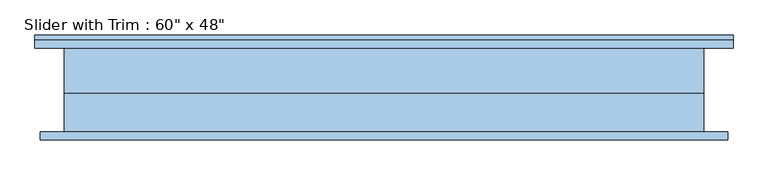
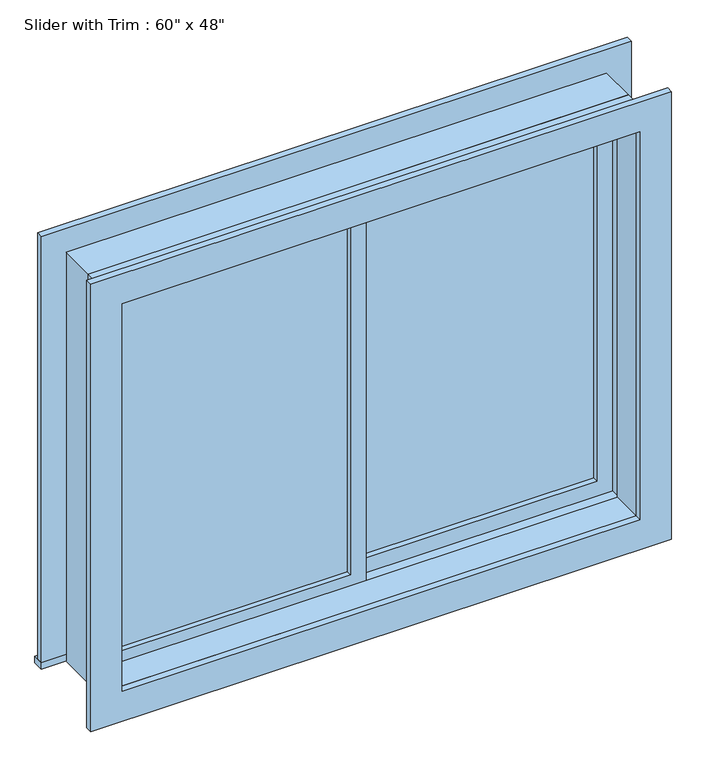
"""IFC4 building model written with IfcOpenShell, lengths in millimetres: window geometry."""

from ifc_helpers import new_model, si_unit, frame, origin, place, context, project, spatial, polyline, outline, extrude, source, transform, mapped, element, save


def window_c4d7a2b1(model_context):
    return source(origin(), model_context, "Body", "SweptSolid", [
        extrude(outline(polyline([(-698.5, 20.625), (-22.225, 20.625), (-22.225, 7.925), (-698.5, 7.925), (-698.5, 20.625)])), frame((0.0, 0.0, 977.9), z_axis=(0.0, 0.0, 1.0), x_axis=(1.0, 0.0, 0.0)), (0.0, 0.0, 1.0), 1092.2),
        extrude(outline(polyline([(2114.55, -742.95), (933.45, -742.95), (933.45, 22.225), (2114.55, 22.225), (2114.55, -742.95)]), holes=[polyline([(2070.1, -698.5), (2070.1, -22.225), (977.9, -22.225), (977.9, -698.5), (2070.1, -698.5)])]), frame((0.0, -7.95, 0.0), z_axis=(0.0, 1.0, 0.0), x_axis=(0.0, 0.0, 1.0)), (0.0, 0.0, 1.0), 44.45),
        extrude(outline(polyline([(-831.85, 131.75), (831.85, 131.75), (831.85, 100.0), (-831.85, 100.0), (-831.85, 131.75)])), frame((0.0, 0.0, 914.4), z_axis=(0.0, 0.0, 1.0), x_axis=(1.0, 0.0, 0.0)), (0.0, 0.0, 1.0), 19.05),
        extrude(outline(polyline([(2114.55, -742.95), (2114.55, 742.95), (933.45, 742.95), (933.45, 831.85), (2203.45, 831.85), (2203.45, -831.85), (933.45, -831.85), (933.45, -742.95), (2114.55, -742.95)])), frame((0.0, 100.0, 0.0), z_axis=(0.0, 1.0, 0.0), x_axis=(0.0, 0.0, 1.0)), (0.0, 0.0, 1.0), 19.05),
        extrude(outline(polyline([(2190.75, 819.15), (2190.75, -819.15), (857.25, -819.15), (857.25, 819.15), (2190.75, 819.15)]), holes=[polyline([(2101.85, 730.25), (946.15, 730.25), (946.15, -730.25), (2101.85, -730.25), (2101.85, 730.25)])]), frame((0.0, -119.05, 0.0), z_axis=(0.0, 1.0, 0.0), x_axis=(0.0, 0.0, 1.0)), (0.0, 0.0, 1.0), 19.05),
        extrude(outline(polyline([(698.5, 52.375), (22.225, 52.375), (22.225, 65.075), (698.5, 65.075), (698.5, 52.375)])), frame((0.0, 0.0, 977.9), z_axis=(0.0, 0.0, 1.0), x_axis=(1.0, 0.0, 0.0)), (0.0, 0.0, 1.0), 1092.2),
        extrude(outline(polyline([(2114.55, -22.225), (933.45, -22.225), (933.45, 742.95), (2114.55, 742.95), (2114.55, -22.225)]), holes=[polyline([(2070.1, 22.225), (2070.1, 698.5), (977.9, 698.5), (977.9, 22.225), (2070.1, 22.225)])]), frame((0.0, 36.5, 0.0), z_axis=(0.0, 1.0, 0.0), x_axis=(0.0, 0.0, 1.0)), (0.0, 0.0, 1.0), 44.45),
        extrude(outline(polyline([(2133.6, -762.0), (914.4, -762.0), (914.4, 762.0), (2133.6, 762.0), (2133.6, -762.0)]), holes=[polyline([(2101.85, -730.25), (2101.85, 730.25), (946.15, 730.25), (946.15, -730.25), (2101.85, -730.25)])]), frame((0.0, -100.0, 0.0), z_axis=(0.0, 1.0, 0.0), x_axis=(0.0, 0.0, 1.0)), (0.0, 0.0, 1.0), 92.05),
        extrude(outline(polyline([(2133.6, 762.0), (2133.6, -762.0), (914.4, -762.0), (914.4, 762.0), (2133.6, 762.0)]), holes=[polyline([(2114.55, 742.95), (933.45, 742.95), (933.45, -742.95), (2114.55, -742.95), (2114.55, 742.95)])]), frame((0.0, -7.95, 0.0), z_axis=(0.0, 1.0, 0.0), x_axis=(0.0, 0.0, 1.0)), (0.0, 0.0, 1.0), 107.95),
    ])


if __name__ == "__main__":
    model = new_model("IFC4")
    model_context = context("Model", 3, world=origin())
    ifc_project = project(units=[si_unit("LENGTHUNIT", "METRE", prefix="MILLI")], contexts=[model_context])
    site = spatial("IfcSite", under=ifc_project)
    building = spatial("IfcBuilding", under=site)
    placement = place(None, origin())
    window_shape = window_c4d7a2b1(model_context)
    element("IfcWindow", 1, ObjectType="Slider with Trim : 60\" x 48\"", at=placement, inside=building, context=model_context, shape_type="MappedRepresentation", body=[
        mapped(window_shape, transform((0.0, 0.0, 0.0), x_axis=(1.0, 0.0, 0.0), y_axis=(0.0, 1.0, 0.0), z_axis=(0.0, 0.0, 1.0))),
    ])
    save(model, "model.ifc")

# Revit data of these elements
# Type "Slider with Trim : 60\" x 48\""
#   Type Mark = "22"
#   Construction Type Id = "GSP4R"
#   Assembly Code = "B2020100"
#   Analytic Construction = "1/8 in Pilkington single glazing"
#   Visual Light Transmittance = 0.9
#   Solar Heat Gain Coefficient = 0.78
#   Heat Transfer Coefficient (U) = 3.6886 W/(m²·K)
#   Height = 4' - 0"
#   Default Sill Height = 3' - 0"
#   Trim Projection - Ext. = 0' - 0 3/4"
#   Trim Projection - Int. = 0' - 0 3/4"
#   Trim Width - Exterior = 0' - 3 1/2"
#   Trim Width - Interior = 0' - 3 1/2"
#   Width = 5' - 0"
#   Window Inset = 0' - 0 3/4"
#   Define Thermal Properties by = 1
#   Glass Pane Material = Glass
#   Sash Material = Sash
#   Trim Exterior Material = Trim
#   Trim Interior Material = Trim
#   Wall Closure = (empty or 0)
# Element 1 (IfcWindow, "Slider with Trim : 60\" x 48\"")
#   Materials on its faces: "Sash", "Trim", "Glass"
# Materials
#   "Glass": class "Glass", colour RGB 218 227 224, transparency 0.85, Description = "Soda Lime Glass", Cost = 0
#   "Sash": class "Wood", colour RGB 136 99 55, transparency 0
#   "Trim": class "Wood", colour RGB 224 178 126, transparency 0
